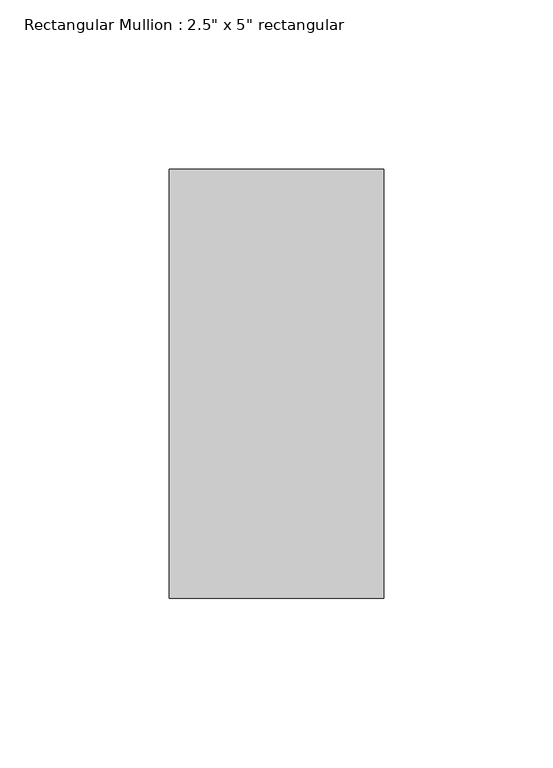
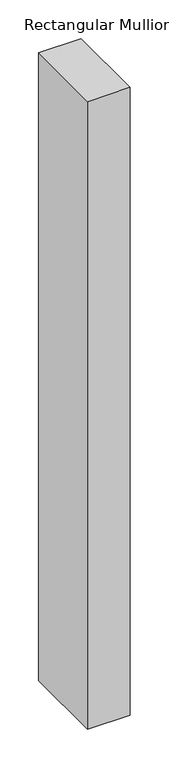
"""IFC4 building model written with IfcOpenShell, lengths in millimetres: member geometry."""

from ifc_helpers import new_model, si_unit, frame, origin, place, context, project, spatial, polyline, outline, extrude, source, transform, mapped, element, save


def member_8f63b531(model_context):
    return source(origin(), model_context, "Body", "SweptSolid", [
        extrude(outline(polyline([(0.0, 63.5), (0.0, -63.5), (-63.5, -63.5), (-63.5, 63.5), (0.0, 63.5)])), frame((0.0, 0.0, -990.6), z_axis=(0.0, 0.0, 1.0), x_axis=(1.0, 0.0, 0.0)), (0.0, 0.0, 1.0), 990.6),
    ])


if __name__ == "__main__":
    model = new_model("IFC4")
    model_context = context("Model", 3, world=origin())
    ifc_project = project(units=[si_unit("LENGTHUNIT", "METRE", prefix="MILLI")], contexts=[model_context])
    site = spatial("IfcSite", under=ifc_project)
    building = spatial("IfcBuilding", under=site)
    placement = place(None, origin())
    member_shape = member_8f63b531(model_context)
    element("IfcMember", 1, ObjectType="Rectangular Mullion : 2.5\" x 5\" rectangular", at=placement, inside=building, context=model_context, shape_type="MappedRepresentation", body=[
        mapped(member_shape, transform((0.0, 0.0, 0.0), x_axis=(1.0, 0.0, 0.0), y_axis=(0.0, 1.0, 0.0), z_axis=(0.0, 0.0, 1.0))),
    ])
    save(model, "model.ifc")

# Revit data of these elements
# Type "Rectangular Mullion : 2.5\" x 5\" rectangular"
#   built-in parameter 1007304 = 0.416667 (stored number, unit not read)
#   built-in parameter 1007301 = 0.104167 (stored number, unit not read)
#   built-in parameter 1007300 = 0.104167 (stored number, unit not read)
# Element 1 (IfcMember, "Rectangular Mullion : 2.5\" x 5\" rectangular")
#   Materials on its faces: "Aluminum"
# Materials
#   "Aluminum": class "Metal", colour RGB 247 247 247, transparency 0, Description = "Aluminum 6061", Cost = 0
